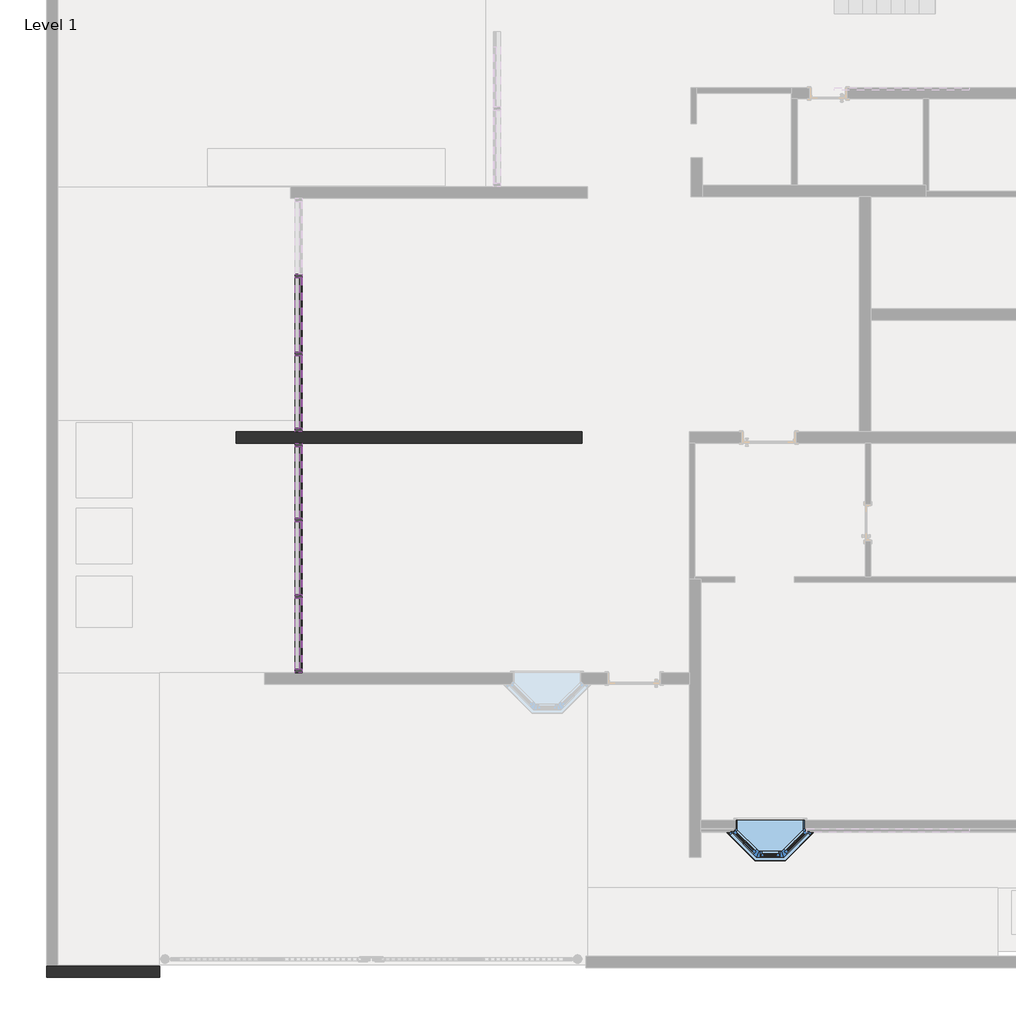
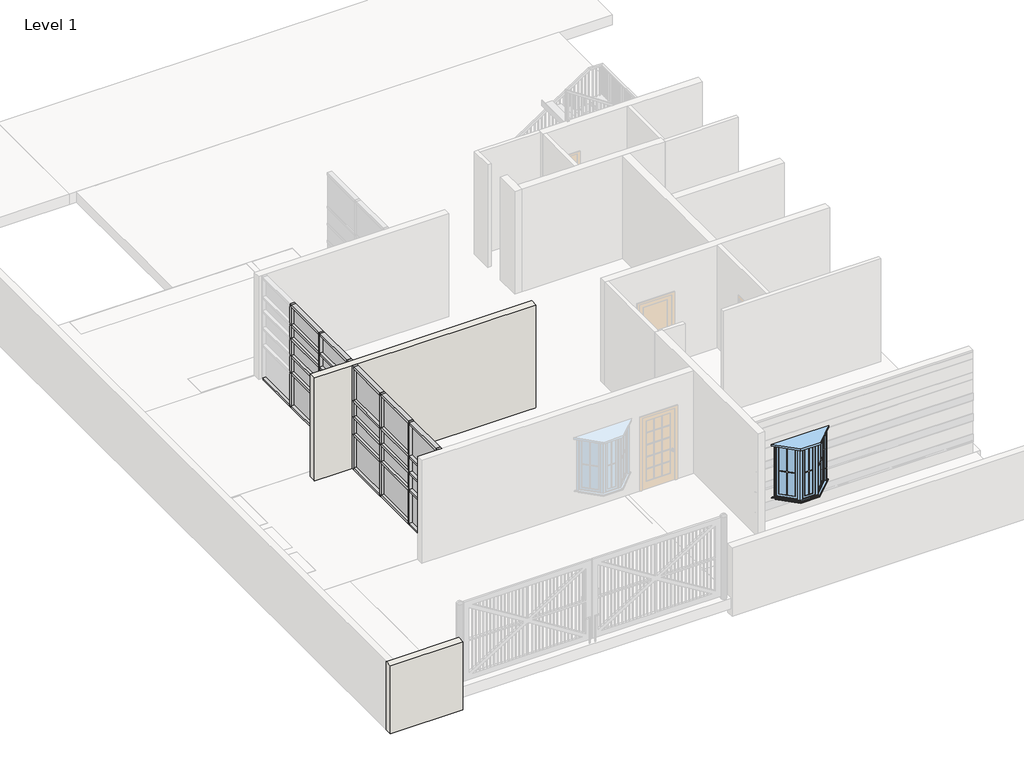
# One storey, part 1 of 5: 59 members, 22 plates, 2 walls, 1 window.
"""IFC4 building model written with IfcOpenShell, lengths in millimetres."""

from ifc_helpers import new_model, si_unit, origin, place, context, project, spatial, faceted_brep, transform, mapped, element, save
from components import member_ace9393b, member_8eff11ef, member_f92b8aa2, member_8e09d03a, member_2b3f0a2a, member_1e564621, member_323df77c, member_86d06fe4, member_556b160f, member_b3098cb3, member_4a65f4ca, member_ce4f90f2, member_13061b82, member_abf390f1, member_37fe5cbd, member_37150780, member_90750a43, member_90c805a2, member_6e77e263, member_47bfaf8a, member_7fd687a9, member_7cfea1b5, system_panel_glazed_a8af599a, system_panel_glazed_c1b4dd64, system_panel_glazed_a0664fa1, system_panel_glazed_cff82037, system_panel_glazed_a94942f9, system_panel_glazed_6f193a35, system_panel_glazed_ac301e25, system_panel_glazed_b1ae2562, system_panel_glazed_b72ced83, system_panel_glazed_3baabbd8, system_panel_glazed_b8338f5c, system_panel_glazed_1cb66d18, system_panel_glazed_2a12a50e, system_panel_glazed_7354da21, system_panel_glazed_2e6a26f2, system_panel_glazed_f09e76d7, window_bay_casement_45_degree_angle_window_4_787d36ed

model = new_model("IFC4")

# Units and contexts
model_context = context("Model", 3, world=origin())
ifc_project = project(units=[si_unit("LENGTHUNIT", "METRE", prefix="MILLI")], contexts=[model_context])

# Site, building, storey
site = spatial("IfcSite", under=ifc_project)
building = spatial("IfcBuilding", under=site)
storey = spatial("IfcBuildingStorey", under=building, Name="Level 1", Elevation=0.0)

# Members
placement = place(None, origin())
member_shape = member_ace9393b(model_context)
element("IfcMember", 1, ObjectType="Rectangular Mullion : 2.5\" x 5\" rectangular", at=placement, inside=storey, context=model_context, shape_type="MappedRepresentation", body=[
    mapped(member_shape, transform((-50759.3380314, -7092.7913973, 3048.0), x_axis=(0.0, 0.0, 1.0), y_axis=(-1.0, 0.0, 0.0), z_axis=(0.0, -1.0, 0.0))),
])
element("IfcMember", 2, ObjectType="Rectangular Mullion : 2.5\" x 5\" rectangular", at=placement, inside=storey, context=model_context, shape_type="MappedRepresentation", body=[
    mapped(member_shape, transform((-50759.3380314, -4381.3413974, 3048.0), x_axis=(0.0, 0.0, 1.0), y_axis=(-1.0, 0.0, 0.0), z_axis=(0.0, -1.0, 0.0))),
])
element("IfcMember", 3, ObjectType="Rectangular Mullion : 2.5\" x 5\" rectangular", at=placement, inside=storey, context=model_context, shape_type="MappedRepresentation", body=[
    mapped(member_shape, transform((-50759.3380314, -3104.9913973, 0.0), x_axis=(0.0, 0.0, -1.0), y_axis=(-1.0, 0.0, 0.0), z_axis=(0.0, 1.0, 0.0))),
])
element("IfcMember", 4, ObjectType="Rectangular Mullion : 2.5\" x 5\" rectangular", at=placement, inside=storey, context=model_context, shape_type="MappedRepresentation", body=[
    mapped(member_shape, transform((-50759.3380314, -5816.4413972, 0.0), x_axis=(0.0, 0.0, -1.0), y_axis=(-1.0, 0.0, 0.0), z_axis=(0.0, 1.0, 0.0))),
])
member_2_shape = member_8eff11ef(model_context)
element("IfcMember", 5, ObjectType="Rectangular Mullion : 2.5\" x 5\" rectangular", at=placement, inside=storey, context=model_context, shape_type="MappedRepresentation", body=[
    mapped(member_2_shape, transform((-50759.3380314, -5752.9413972, 3048.0), x_axis=(0.0, 0.0, 1.0), y_axis=(-1.0, 0.0, 0.0), z_axis=(0.0, -1.0, 0.0))),
])
element("IfcMember", 6, ObjectType="Rectangular Mullion : 2.5\" x 5\" rectangular", at=placement, inside=storey, context=model_context, shape_type="MappedRepresentation", body=[
    mapped(member_2_shape, transform((-50759.3380314, -4444.8413974, 0.0), x_axis=(0.0, 0.0, -1.0), y_axis=(-1.0, 0.0, 0.0), z_axis=(0.0, 1.0, 0.0))),
])
member_3_shape = member_f92b8aa2(model_context)
element("IfcMember", 7, ObjectType="Rectangular Mullion : 2.5\" x 5\" rectangular", at=placement, inside=storey, context=model_context, shape_type="MappedRepresentation", body=[
    mapped(member_3_shape, transform((-50759.3380314, -4413.0913974, 2032.0), x_axis=(0.0, -1.0, 0.0), y_axis=(-1.0, 0.0, 0.0), z_axis=(0.0, 0.0, -1.0))),
])
element("IfcMember", 8, ObjectType="Rectangular Mullion : 2.5\" x 5\" rectangular", at=placement, inside=storey, context=model_context, shape_type="MappedRepresentation", body=[
    mapped(member_3_shape, transform((-50759.3380314, -5784.6913972, 2032.0), x_axis=(0.0, -1.0, 0.0), y_axis=(-1.0, 0.0, 0.0), z_axis=(0.0, 0.0, -1.0))),
])
member_4_shape = member_8e09d03a(model_context)
element("IfcMember", 9, ObjectType="Rectangular Mullion : 2.5\" x 5\" rectangular", at=placement, inside=storey, context=model_context, shape_type="MappedRepresentation", body=[
    mapped(member_4_shape, transform((-50759.3380314, -3041.4913973, 3048.0), x_axis=(0.0, 1.0, 0.0), y_axis=(-1.0, 0.0, 0.0), z_axis=(0.0, 0.0, 1.0))),
])
element("IfcMember", 10, ObjectType="Rectangular Mullion : 2.5\" x 5\" rectangular", at=placement, inside=storey, context=model_context, shape_type="MappedRepresentation", body=[
    mapped(member_4_shape, transform((-50759.3380314, -7156.2913973, 2032.0), x_axis=(0.0, -1.0, 0.0), y_axis=(-1.0, 0.0, 0.0), z_axis=(0.0, 0.0, -1.0))),
])
member_5_shape = member_2b3f0a2a(model_context)
element("IfcMember", 11, ObjectType="Rectangular Mullion : 2.5\" x 5\" rectangular", at=placement, inside=storey, context=model_context, shape_type="MappedRepresentation", body=[
    mapped(member_5_shape, transform((-50759.3380314, -4381.3413974, 2032.0), x_axis=(0.0, 0.0, 1.0), y_axis=(-1.0, 0.0, 0.0), z_axis=(0.0, -1.0, 0.0))),
])
element("IfcMember", 12, ObjectType="Rectangular Mullion : 2.5\" x 5\" rectangular", at=placement, inside=storey, context=model_context, shape_type="MappedRepresentation", body=[
    mapped(member_5_shape, transform((-50759.3380314, -7092.7913973, 2032.0), x_axis=(0.0, 0.0, 1.0), y_axis=(-1.0, 0.0, 0.0), z_axis=(0.0, -1.0, 0.0))),
])
element("IfcMember", 13, ObjectType="Rectangular Mullion : 2.5\" x 5\" rectangular", at=placement, inside=storey, context=model_context, shape_type="MappedRepresentation", body=[
    mapped(member_5_shape, transform((-50759.3380314, -4381.3413974, 1549.4), x_axis=(0.0, 0.0, 1.0), y_axis=(-1.0, 0.0, 0.0), z_axis=(0.0, -1.0, 0.0))),
])
element("IfcMember", 14, ObjectType="Rectangular Mullion : 2.5\" x 5\" rectangular", at=placement, inside=storey, context=model_context, shape_type="MappedRepresentation", body=[
    mapped(member_5_shape, transform((-50759.3380314, -7092.7913973, 1549.4), x_axis=(0.0, 0.0, 1.0), y_axis=(-1.0, 0.0, 0.0), z_axis=(0.0, -1.0, 0.0))),
])
element("IfcMember", 15, ObjectType="Rectangular Mullion : 2.5\" x 5\" rectangular", at=placement, inside=storey, context=model_context, shape_type="MappedRepresentation", body=[
    mapped(member_5_shape, transform((-50759.3380314, -4381.3413974, 1032.9333333), x_axis=(0.0, 0.0, 1.0), y_axis=(-1.0, 0.0, 0.0), z_axis=(0.0, -1.0, 0.0))),
])
element("IfcMember", 16, ObjectType="Rectangular Mullion : 2.5\" x 5\" rectangular", at=placement, inside=storey, context=model_context, shape_type="MappedRepresentation", body=[
    mapped(member_5_shape, transform((-50759.3380314, -7092.7913973, 1032.9333333), x_axis=(0.0, 0.0, 1.0), y_axis=(-1.0, 0.0, 0.0), z_axis=(0.0, -1.0, 0.0))),
])
member_6_shape = member_1e564621(model_context)
element("IfcMember", 17, ObjectType="Rectangular Mullion : 2.5\" x 5\" rectangular", at=placement, inside=storey, context=model_context, shape_type="MappedRepresentation", body=[
    mapped(member_6_shape, transform((-50759.3380314, -5752.9413972, 2032.0), x_axis=(0.0, 0.0, 1.0), y_axis=(-1.0, 0.0, 0.0), z_axis=(0.0, -1.0, 0.0))),
])
element("IfcMember", 18, ObjectType="Rectangular Mullion : 2.5\" x 5\" rectangular", at=placement, inside=storey, context=model_context, shape_type="MappedRepresentation", body=[
    mapped(member_6_shape, transform((-50759.3380314, -5752.9413972, 1549.4), x_axis=(0.0, 0.0, 1.0), y_axis=(-1.0, 0.0, 0.0), z_axis=(0.0, -1.0, 0.0))),
])
element("IfcMember", 19, ObjectType="Rectangular Mullion : 2.5\" x 5\" rectangular", at=placement, inside=storey, context=model_context, shape_type="MappedRepresentation", body=[
    mapped(member_6_shape, transform((-50759.3380314, -5752.9413972, 1032.9333333), x_axis=(0.0, 0.0, 1.0), y_axis=(-1.0, 0.0, 0.0), z_axis=(0.0, -1.0, 0.0))),
])
member_7_shape = member_323df77c(model_context)
element("IfcMember", 20, ObjectType="Rectangular Mullion : 2.5\" x 5\" rectangular", at=placement, inside=storey, context=model_context, shape_type="MappedRepresentation", body=[
    mapped(member_7_shape, transform((-50759.3380314, -4413.0913974, 1549.4), x_axis=(0.0, -1.0, 0.0), y_axis=(-1.0, 0.0, 0.0), z_axis=(0.0, 0.0, -1.0))),
])
element("IfcMember", 21, ObjectType="Rectangular Mullion : 2.5\" x 5\" rectangular", at=placement, inside=storey, context=model_context, shape_type="MappedRepresentation", body=[
    mapped(member_7_shape, transform((-50759.3380314, -5784.6913972, 1549.4), x_axis=(0.0, -1.0, 0.0), y_axis=(-1.0, 0.0, 0.0), z_axis=(0.0, 0.0, -1.0))),
])
member_8_shape = member_86d06fe4(model_context)
element("IfcMember", 22, ObjectType="Rectangular Mullion : 2.5\" x 5\" rectangular", at=placement, inside=storey, context=model_context, shape_type="MappedRepresentation", body=[
    mapped(member_8_shape, transform((-50759.3380314, -3041.4913973, 2032.0), x_axis=(0.0, 1.0, 0.0), y_axis=(-1.0, 0.0, 0.0), z_axis=(0.0, 0.0, 1.0))),
])
element("IfcMember", 23, ObjectType="Rectangular Mullion : 2.5\" x 5\" rectangular", at=placement, inside=storey, context=model_context, shape_type="MappedRepresentation", body=[
    mapped(member_8_shape, transform((-50759.3380314, -7156.2913973, 1549.4), x_axis=(0.0, -1.0, 0.0), y_axis=(-1.0, 0.0, 0.0), z_axis=(0.0, 0.0, -1.0))),
])
member_9_shape = member_556b160f(model_context)
element("IfcMember", 24, ObjectType="Rectangular Mullion : 2.5\" x 5\" rectangular", at=placement, inside=storey, context=model_context, shape_type="MappedRepresentation", body=[
    mapped(member_9_shape, transform((-50759.3380314, -4413.0913974, 0.0), x_axis=(0.0, -1.0, 0.0), y_axis=(-1.0, 0.0, 0.0), z_axis=(0.0, 0.0, -1.0))),
])
element("IfcMember", 25, ObjectType="Rectangular Mullion : 2.5\" x 5\" rectangular", at=placement, inside=storey, context=model_context, shape_type="MappedRepresentation", body=[
    mapped(member_9_shape, transform((-50759.3380314, -5784.6913972, 0.0), x_axis=(0.0, -1.0, 0.0), y_axis=(-1.0, 0.0, 0.0), z_axis=(0.0, 0.0, -1.0))),
])
member_10_shape = member_b3098cb3(model_context)
element("IfcMember", 26, ObjectType="Rectangular Mullion : 2.5\" x 5\" rectangular", at=placement, inside=storey, context=model_context, shape_type="MappedRepresentation", body=[
    mapped(member_10_shape, transform((-50759.3380314, -4413.0913974, 1032.9333333), x_axis=(0.0, -1.0, 0.0), y_axis=(-1.0, 0.0, 0.0), z_axis=(0.0, 0.0, -1.0))),
])
element("IfcMember", 27, ObjectType="Rectangular Mullion : 2.5\" x 5\" rectangular", at=placement, inside=storey, context=model_context, shape_type="MappedRepresentation", body=[
    mapped(member_10_shape, transform((-50759.3380314, -5784.6913972, 1032.9333333), x_axis=(0.0, -1.0, 0.0), y_axis=(-1.0, 0.0, 0.0), z_axis=(0.0, 0.0, -1.0))),
])
member_11_shape = member_4a65f4ca(model_context)
element("IfcMember", 28, ObjectType="Rectangular Mullion : 2.5\" x 5\" rectangular", at=placement, inside=storey, context=model_context, shape_type="MappedRepresentation", body=[
    mapped(member_11_shape, transform((-50759.3380314, -7156.2913973, 0.0), x_axis=(0.0, -1.0, 0.0), y_axis=(-1.0, 0.0, 0.0), z_axis=(0.0, 0.0, -1.0))),
])
member_12_shape = member_ce4f90f2(model_context)
element("IfcMember", 29, ObjectType="Rectangular Mullion : 2.5\" x 5\" rectangular", at=placement, inside=storey, context=model_context, shape_type="MappedRepresentation", body=[
    mapped(member_12_shape, transform((-50759.3380314, -3041.4913973, 1549.4), x_axis=(0.0, 1.0, 0.0), y_axis=(-1.0, 0.0, 0.0), z_axis=(0.0, 0.0, 1.0))),
])
element("IfcMember", 30, ObjectType="Rectangular Mullion : 2.5\" x 5\" rectangular", at=placement, inside=storey, context=model_context, shape_type="MappedRepresentation", body=[
    mapped(member_12_shape, transform((-50759.3380314, -7156.2913973, 1032.9333333), x_axis=(0.0, -1.0, 0.0), y_axis=(-1.0, 0.0, 0.0), z_axis=(0.0, 0.0, -1.0))),
])
element("IfcMember", 31, ObjectType="Rectangular Mullion : 2.5\" x 5\" rectangular", at=placement, inside=storey, context=model_context, shape_type="MappedRepresentation", body=[
    mapped(member_11_shape, transform((-50759.3380314, -3041.4913973, 1032.9333333), x_axis=(0.0, 1.0, 0.0), y_axis=(-1.0, 0.0, 0.0), z_axis=(0.0, 0.0, 1.0))),
])
member_13_shape = member_13061b82(model_context)
element("IfcMember", 32, ObjectType="Rectangular Mullion : 2.5\" x 5\" rectangular", at=placement, inside=storey, context=model_context, shape_type="MappedRepresentation", body=[
    mapped(member_13_shape, transform((-50759.3380314, -1473.0413972, 3048.0), x_axis=(0.0, 0.0, 1.0), y_axis=(1.0, 0.0, 0.0), z_axis=(0.0, 1.0, 0.0))),
])
element("IfcMember", 33, ObjectType="Rectangular Mullion : 2.5\" x 5\" rectangular", at=placement, inside=storey, context=model_context, shape_type="MappedRepresentation", body=[
    mapped(member_13_shape, transform((-50759.3380314, -2774.7913973, 0.0), x_axis=(0.0, 0.0, -1.0), y_axis=(1.0, 0.0, 0.0), z_axis=(0.0, -1.0, 0.0))),
])
element("IfcMember", 34, ObjectType="Rectangular Mullion : 2.5\" x 5\" rectangular", at=placement, inside=storey, context=model_context, shape_type="MappedRepresentation", body=[
    mapped(member_13_shape, transform((-50759.3380314, -12.5413974, 0.0), x_axis=(0.0, 0.0, -1.0), y_axis=(1.0, 0.0, 0.0), z_axis=(0.0, -1.0, 0.0))),
])
member_14_shape = member_abf390f1(model_context)
element("IfcMember", 35, ObjectType="Rectangular Mullion : 2.5\" x 5\" rectangular", at=placement, inside=storey, context=model_context, shape_type="MappedRepresentation", body=[
    mapped(member_14_shape, transform((-50759.3380314, -76.0413974, 3048.0), x_axis=(0.0, 0.0, 1.0), y_axis=(1.0, 0.0, 0.0), z_axis=(0.0, 1.0, 0.0))),
])
element("IfcMember", 36, ObjectType="Rectangular Mullion : 2.5\" x 5\" rectangular", at=placement, inside=storey, context=model_context, shape_type="MappedRepresentation", body=[
    mapped(member_14_shape, transform((-50759.3380314, -1409.5413972, 0.0), x_axis=(0.0, 0.0, -1.0), y_axis=(1.0, 0.0, 0.0), z_axis=(0.0, -1.0, 0.0))),
])
element("IfcMember", 37, ObjectType="Rectangular Mullion : 2.5\" x 5\" rectangular", at=placement, inside=storey, context=model_context, shape_type="MappedRepresentation", body=[
    mapped(member_3_shape, transform((-50759.3380314, -1441.2913972, 0.0), x_axis=(0.0, 1.0, 0.0), y_axis=(1.0, 0.0, 0.0), z_axis=(0.0, 0.0, -1.0))),
])
element("IfcMember", 38, ObjectType="Rectangular Mullion : 2.5\" x 5\" rectangular", at=placement, inside=storey, context=model_context, shape_type="MappedRepresentation", body=[
    mapped(member_3_shape, transform((-50759.3380314, -44.2913974, 0.0), x_axis=(0.0, 1.0, 0.0), y_axis=(1.0, 0.0, 0.0), z_axis=(0.0, 0.0, -1.0))),
])
member_15_shape = member_37fe5cbd(model_context)
element("IfcMember", 39, ObjectType="Rectangular Mullion : 2.5\" x 5\" rectangular", at=placement, inside=storey, context=model_context, shape_type="MappedRepresentation", body=[
    mapped(member_15_shape, transform((-50759.3380314, -1473.0413972, 1016.0), x_axis=(0.0, 0.0, 1.0), y_axis=(1.0, 0.0, 0.0), z_axis=(0.0, 1.0, 0.0))),
])
element("IfcMember", 40, ObjectType="Rectangular Mullion : 2.5\" x 5\" rectangular", at=placement, inside=storey, context=model_context, shape_type="MappedRepresentation", body=[
    mapped(member_15_shape, transform((-50759.3380314, -1473.0413972, 2032.0), x_axis=(0.0, 0.0, 1.0), y_axis=(1.0, 0.0, 0.0), z_axis=(0.0, 1.0, 0.0))),
])
element("IfcMember", 41, ObjectType="Rectangular Mullion : 2.5\" x 5\" rectangular", at=placement, inside=storey, context=model_context, shape_type="MappedRepresentation", body=[
    mapped(member_15_shape, transform((-50759.3380314, -1473.0413972, 1524.0), x_axis=(0.0, 0.0, 1.0), y_axis=(1.0, 0.0, 0.0), z_axis=(0.0, 1.0, 0.0))),
])
element("IfcMember", 42, ObjectType="Rectangular Mullion : 2.5\" x 5\" rectangular", at=placement, inside=storey, context=model_context, shape_type="MappedRepresentation", body=[
    mapped(member_15_shape, transform((-50759.3380314, -1473.0413972, 2438.4), x_axis=(0.0, 0.0, 1.0), y_axis=(1.0, 0.0, 0.0), z_axis=(0.0, 1.0, 0.0))),
])
member_16_shape = member_37150780(model_context)
element("IfcMember", 43, ObjectType="Rectangular Mullion : 2.5\" x 5\" rectangular", at=placement, inside=storey, context=model_context, shape_type="MappedRepresentation", body=[
    mapped(member_16_shape, transform((-50759.3380314, -76.0413974, 1016.0), x_axis=(0.0, 0.0, 1.0), y_axis=(1.0, 0.0, 0.0), z_axis=(0.0, 1.0, 0.0))),
])
element("IfcMember", 44, ObjectType="Rectangular Mullion : 2.5\" x 5\" rectangular", at=placement, inside=storey, context=model_context, shape_type="MappedRepresentation", body=[
    mapped(member_16_shape, transform((-50759.3380314, -76.0413974, 2032.0), x_axis=(0.0, 0.0, 1.0), y_axis=(1.0, 0.0, 0.0), z_axis=(0.0, 1.0, 0.0))),
])
element("IfcMember", 45, ObjectType="Rectangular Mullion : 2.5\" x 5\" rectangular", at=placement, inside=storey, context=model_context, shape_type="MappedRepresentation", body=[
    mapped(member_16_shape, transform((-50759.3380314, -76.0413974, 1524.0), x_axis=(0.0, 0.0, 1.0), y_axis=(1.0, 0.0, 0.0), z_axis=(0.0, 1.0, 0.0))),
])
element("IfcMember", 46, ObjectType="Rectangular Mullion : 2.5\" x 5\" rectangular", at=placement, inside=storey, context=model_context, shape_type="MappedRepresentation", body=[
    mapped(member_16_shape, transform((-50759.3380314, -76.0413974, 2438.4), x_axis=(0.0, 0.0, 1.0), y_axis=(1.0, 0.0, 0.0), z_axis=(0.0, 1.0, 0.0))),
])
member_17_shape = member_90750a43(model_context)
element("IfcMember", 47, ObjectType="Rectangular Mullion : 2.5\" x 5\" rectangular", at=placement, inside=storey, context=model_context, shape_type="MappedRepresentation", body=[
    mapped(member_17_shape, transform((-50759.3380314, -1441.2913972, 1016.0), x_axis=(0.0, 1.0, 0.0), y_axis=(1.0, 0.0, 0.0), z_axis=(0.0, 0.0, -1.0))),
])
element("IfcMember", 48, ObjectType="Rectangular Mullion : 2.5\" x 5\" rectangular", at=placement, inside=storey, context=model_context, shape_type="MappedRepresentation", body=[
    mapped(member_17_shape, transform((-50759.3380314, -44.2913974, 1016.0), x_axis=(0.0, 1.0, 0.0), y_axis=(1.0, 0.0, 0.0), z_axis=(0.0, 0.0, -1.0))),
])
element("IfcMember", 49, ObjectType="Rectangular Mullion : 2.5\" x 5\" rectangular", at=placement, inside=storey, context=model_context, shape_type="MappedRepresentation", body=[
    mapped(member_17_shape, transform((-50759.3380314, -1441.2913972, 1524.0), x_axis=(0.0, 1.0, 0.0), y_axis=(1.0, 0.0, 0.0), z_axis=(0.0, 0.0, -1.0))),
])
element("IfcMember", 50, ObjectType="Rectangular Mullion : 2.5\" x 5\" rectangular", at=placement, inside=storey, context=model_context, shape_type="MappedRepresentation", body=[
    mapped(member_17_shape, transform((-50759.3380314, -44.2913974, 1524.0), x_axis=(0.0, 1.0, 0.0), y_axis=(1.0, 0.0, 0.0), z_axis=(0.0, 0.0, -1.0))),
])
member_18_shape = member_90c805a2(model_context)
element("IfcMember", 51, ObjectType="Rectangular Mullion : 2.5\" x 5\" rectangular", at=placement, inside=storey, context=model_context, shape_type="MappedRepresentation", body=[
    mapped(member_18_shape, transform((-50759.3380314, -1441.2913972, 2032.0), x_axis=(0.0, 1.0, 0.0), y_axis=(1.0, 0.0, 0.0), z_axis=(0.0, 0.0, -1.0))),
])
element("IfcMember", 52, ObjectType="Rectangular Mullion : 2.5\" x 5\" rectangular", at=placement, inside=storey, context=model_context, shape_type="MappedRepresentation", body=[
    mapped(member_18_shape, transform((-50759.3380314, -44.2913974, 2032.0), x_axis=(0.0, 1.0, 0.0), y_axis=(1.0, 0.0, 0.0), z_axis=(0.0, 0.0, -1.0))),
])
member_19_shape = member_6e77e263(model_context)
element("IfcMember", 53, ObjectType="Rectangular Mullion : 2.5\" x 5\" rectangular", at=placement, inside=storey, context=model_context, shape_type="MappedRepresentation", body=[
    mapped(member_19_shape, transform((-50759.3380314, -1441.2913972, 2438.4), x_axis=(0.0, 1.0, 0.0), y_axis=(1.0, 0.0, 0.0), z_axis=(0.0, 0.0, -1.0))),
])
element("IfcMember", 54, ObjectType="Rectangular Mullion : 2.5\" x 5\" rectangular", at=placement, inside=storey, context=model_context, shape_type="MappedRepresentation", body=[
    mapped(member_19_shape, transform((-50759.3380314, -44.2913974, 2438.4), x_axis=(0.0, 1.0, 0.0), y_axis=(1.0, 0.0, 0.0), z_axis=(0.0, 0.0, -1.0))),
])
member_20_shape = member_47bfaf8a(model_context)
element("IfcMember", 55, ObjectType="Rectangular Mullion : 2.5\" x 5\" rectangular", at=placement, inside=storey, context=model_context, shape_type="MappedRepresentation", body=[
    mapped(member_20_shape, transform((-50759.3380314, -2838.2913973, 3048.0), x_axis=(0.0, -1.0, 0.0), y_axis=(1.0, 0.0, 0.0), z_axis=(0.0, 0.0, 1.0))),
])
element("IfcMember", 56, ObjectType="Rectangular Mullion : 2.5\" x 5\" rectangular", at=placement, inside=storey, context=model_context, shape_type="MappedRepresentation", body=[
    mapped(member_4_shape, transform((-50759.3380314, -2838.2913973, 1016.0), x_axis=(0.0, -1.0, 0.0), y_axis=(1.0, 0.0, 0.0), z_axis=(0.0, 0.0, 1.0))),
])
member_21_shape = member_7fd687a9(model_context)
element("IfcMember", 57, ObjectType="Rectangular Mullion : 2.5\" x 5\" rectangular", at=placement, inside=storey, context=model_context, shape_type="MappedRepresentation", body=[
    mapped(member_21_shape, transform((-50759.3380314, -2838.2913973, 2032.0), x_axis=(0.0, -1.0, 0.0), y_axis=(1.0, 0.0, 0.0), z_axis=(0.0, 0.0, 1.0))),
])
element("IfcMember", 58, ObjectType="Rectangular Mullion : 2.5\" x 5\" rectangular", at=placement, inside=storey, context=model_context, shape_type="MappedRepresentation", body=[
    mapped(member_21_shape, transform((-50759.3380314, -2838.2913973, 1524.0), x_axis=(0.0, -1.0, 0.0), y_axis=(1.0, 0.0, 0.0), z_axis=(0.0, 0.0, 1.0))),
])
member_22_shape = member_7cfea1b5(model_context)
element("IfcMember", 59, ObjectType="Rectangular Mullion : 2.5\" x 5\" rectangular", at=placement, inside=storey, context=model_context, shape_type="MappedRepresentation", body=[
    mapped(member_22_shape, transform((-50759.3380314, -2838.2913973, 2438.4), x_axis=(0.0, -1.0, 0.0), y_axis=(1.0, 0.0, 0.0), z_axis=(0.0, 0.0, 1.0))),
])

# Plates
system_panel_glazed_shape = system_panel_glazed_a8af599a(model_context)
element("IfcPlate", 60, ObjectType="System Panel : Glazed", at=placement, inside=storey, context=model_context, shape_type="MappedRepresentation", body=[
    mapped(system_panel_glazed_shape, transform((-50759.3380314, -3743.1663973, 2063.75), x_axis=(0.0, -1.0, 0.0), y_axis=(1.0, 0.0, 0.0), z_axis=(0.0, 0.0, 1.0))),
])
element("IfcPlate", 61, ObjectType="System Panel : Glazed", at=placement, inside=storey, context=model_context, shape_type="MappedRepresentation", body=[
    mapped(system_panel_glazed_shape, transform((-50759.3380314, -6454.6163972, 2063.75), x_axis=(0.0, -1.0, 0.0), y_axis=(1.0, 0.0, 0.0), z_axis=(0.0, 0.0, 1.0))),
])
system_panel_glazed_2_shape = system_panel_glazed_c1b4dd64(model_context)
element("IfcPlate", 62, ObjectType="System Panel : Glazed", at=placement, inside=storey, context=model_context, shape_type="MappedRepresentation", body=[
    mapped(system_panel_glazed_2_shape, transform((-50759.3380314, -5098.8913973, 2063.75), x_axis=(0.0, -1.0, 0.0), y_axis=(1.0, 0.0, 0.0), z_axis=(0.0, 0.0, 1.0))),
])
system_panel_glazed_3_shape = system_panel_glazed_a0664fa1(model_context)
element("IfcPlate", 63, ObjectType="System Panel : Glazed", at=placement, inside=storey, context=model_context, shape_type="MappedRepresentation", body=[
    mapped(system_panel_glazed_3_shape, transform((-50759.3380314, -3743.1663973, 1581.15), x_axis=(0.0, -1.0, 0.0), y_axis=(1.0, 0.0, 0.0), z_axis=(0.0, 0.0, 1.0))),
])
element("IfcPlate", 64, ObjectType="System Panel : Glazed", at=placement, inside=storey, context=model_context, shape_type="MappedRepresentation", body=[
    mapped(system_panel_glazed_3_shape, transform((-50759.3380314, -6454.6163972, 1581.15), x_axis=(0.0, -1.0, 0.0), y_axis=(1.0, 0.0, 0.0), z_axis=(0.0, 0.0, 1.0))),
])
system_panel_glazed_4_shape = system_panel_glazed_cff82037(model_context)
element("IfcPlate", 65, ObjectType="System Panel : Glazed", at=placement, inside=storey, context=model_context, shape_type="MappedRepresentation", body=[
    mapped(system_panel_glazed_4_shape, transform((-50759.3380314, -5098.8913973, 1581.15), x_axis=(0.0, -1.0, 0.0), y_axis=(1.0, 0.0, 0.0), z_axis=(0.0, 0.0, 1.0))),
])
system_panel_glazed_5_shape = system_panel_glazed_a94942f9(model_context)
element("IfcPlate", 66, ObjectType="System Panel : Glazed", at=placement, inside=storey, context=model_context, shape_type="MappedRepresentation", body=[
    mapped(system_panel_glazed_5_shape, transform((-50759.3380314, -3743.1663973, 63.5), x_axis=(0.0, -1.0, 0.0), y_axis=(1.0, 0.0, 0.0), z_axis=(0.0, 0.0, 1.0))),
])
element("IfcPlate", 67, ObjectType="System Panel : Glazed", at=placement, inside=storey, context=model_context, shape_type="MappedRepresentation", body=[
    mapped(system_panel_glazed_5_shape, transform((-50759.3380314, -6454.6163972, 63.5), x_axis=(0.0, -1.0, 0.0), y_axis=(1.0, 0.0, 0.0), z_axis=(0.0, 0.0, 1.0))),
])
system_panel_glazed_6_shape = system_panel_glazed_6f193a35(model_context)
element("IfcPlate", 68, ObjectType="System Panel : Glazed", at=placement, inside=storey, context=model_context, shape_type="MappedRepresentation", body=[
    mapped(system_panel_glazed_6_shape, transform((-50759.3380314, -5098.8913973, 63.5), x_axis=(0.0, -1.0, 0.0), y_axis=(1.0, 0.0, 0.0), z_axis=(0.0, 0.0, 1.0))),
])
system_panel_glazed_7_shape = system_panel_glazed_ac301e25(model_context)
element("IfcPlate", 69, ObjectType="System Panel : Glazed", at=placement, inside=storey, context=model_context, shape_type="MappedRepresentation", body=[
    mapped(system_panel_glazed_7_shape, transform((-50759.3380314, -3743.1663973, 1064.6833333), x_axis=(0.0, -1.0, 0.0), y_axis=(1.0, 0.0, 0.0), z_axis=(0.0, 0.0, 1.0))),
])
element("IfcPlate", 70, ObjectType="System Panel : Glazed", at=placement, inside=storey, context=model_context, shape_type="MappedRepresentation", body=[
    mapped(system_panel_glazed_7_shape, transform((-50759.3380314, -6454.6163972, 1064.6833333), x_axis=(0.0, -1.0, 0.0), y_axis=(1.0, 0.0, 0.0), z_axis=(0.0, 0.0, 1.0))),
])
system_panel_glazed_8_shape = system_panel_glazed_b1ae2562(model_context)
element("IfcPlate", 71, ObjectType="System Panel : Glazed", at=placement, inside=storey, context=model_context, shape_type="MappedRepresentation", body=[
    mapped(system_panel_glazed_8_shape, transform((-50759.3380314, -5098.8913973, 1064.6833333), x_axis=(0.0, -1.0, 0.0), y_axis=(1.0, 0.0, 0.0), z_axis=(0.0, 0.0, 1.0))),
])
system_panel_glazed_9_shape = system_panel_glazed_b72ced83(model_context)
element("IfcPlate", 72, ObjectType="System Panel : Glazed", at=placement, inside=storey, context=model_context, shape_type="MappedRepresentation", body=[
    mapped(system_panel_glazed_9_shape, transform((-50759.3380314, -2123.9163972, 63.5), x_axis=(0.0, 1.0, 0.0), y_axis=(-1.0, 0.0, 0.0), z_axis=(0.0, 0.0, 1.0))),
])
system_panel_glazed_10_shape = system_panel_glazed_3baabbd8(model_context)
element("IfcPlate", 73, ObjectType="System Panel : Glazed", at=placement, inside=storey, context=model_context, shape_type="MappedRepresentation", body=[
    mapped(system_panel_glazed_10_shape, transform((-50759.3380314, -742.7913973, 63.5), x_axis=(0.0, 1.0, 0.0), y_axis=(-1.0, 0.0, 0.0), z_axis=(0.0, 0.0, 1.0))),
])
system_panel_glazed_11_shape = system_panel_glazed_b8338f5c(model_context)
element("IfcPlate", 74, ObjectType="System Panel : Glazed", at=placement, inside=storey, context=model_context, shape_type="MappedRepresentation", body=[
    mapped(system_panel_glazed_11_shape, transform((-50759.3380314, -2123.9163972, 1047.75), x_axis=(0.0, 1.0, 0.0), y_axis=(-1.0, 0.0, 0.0), z_axis=(0.0, 0.0, 1.0))),
])
element("IfcPlate", 75, ObjectType="System Panel : Glazed", at=placement, inside=storey, context=model_context, shape_type="MappedRepresentation", body=[
    mapped(system_panel_glazed_11_shape, transform((-50759.3380314, -2123.9163972, 1555.75), x_axis=(0.0, 1.0, 0.0), y_axis=(-1.0, 0.0, 0.0), z_axis=(0.0, 0.0, 1.0))),
])
system_panel_glazed_12_shape = system_panel_glazed_1cb66d18(model_context)
element("IfcPlate", 76, ObjectType="System Panel : Glazed", at=placement, inside=storey, context=model_context, shape_type="MappedRepresentation", body=[
    mapped(system_panel_glazed_12_shape, transform((-50759.3380314, -742.7913973, 1047.75), x_axis=(0.0, 1.0, 0.0), y_axis=(-1.0, 0.0, 0.0), z_axis=(0.0, 0.0, 1.0))),
])
element("IfcPlate", 77, ObjectType="System Panel : Glazed", at=placement, inside=storey, context=model_context, shape_type="MappedRepresentation", body=[
    mapped(system_panel_glazed_12_shape, transform((-50759.3380314, -742.7913973, 1555.75), x_axis=(0.0, 1.0, 0.0), y_axis=(-1.0, 0.0, 0.0), z_axis=(0.0, 0.0, 1.0))),
])
system_panel_glazed_13_shape = system_panel_glazed_2a12a50e(model_context)
element("IfcPlate", 78, ObjectType="System Panel : Glazed", at=placement, inside=storey, context=model_context, shape_type="MappedRepresentation", body=[
    mapped(system_panel_glazed_13_shape, transform((-50759.3380314, -2123.9163972, 2063.75), x_axis=(0.0, 1.0, 0.0), y_axis=(-1.0, 0.0, 0.0), z_axis=(0.0, 0.0, 1.0))),
])
system_panel_glazed_14_shape = system_panel_glazed_7354da21(model_context)
element("IfcPlate", 79, ObjectType="System Panel : Glazed", at=placement, inside=storey, context=model_context, shape_type="MappedRepresentation", body=[
    mapped(system_panel_glazed_14_shape, transform((-50759.3380314, -742.7913973, 2063.75), x_axis=(0.0, 1.0, 0.0), y_axis=(-1.0, 0.0, 0.0), z_axis=(0.0, 0.0, 1.0))),
])
system_panel_glazed_15_shape = system_panel_glazed_2e6a26f2(model_context)
element("IfcPlate", 80, ObjectType="System Panel : Glazed", at=placement, inside=storey, context=model_context, shape_type="MappedRepresentation", body=[
    mapped(system_panel_glazed_15_shape, transform((-50759.3380314, -2123.9163972, 2470.15), x_axis=(0.0, 1.0, 0.0), y_axis=(-1.0, 0.0, 0.0), z_axis=(0.0, 0.0, 1.0))),
])
system_panel_glazed_16_shape = system_panel_glazed_f09e76d7(model_context)
element("IfcPlate", 81, ObjectType="System Panel : Glazed", at=placement, inside=storey, context=model_context, shape_type="MappedRepresentation", body=[
    mapped(system_panel_glazed_16_shape, transform((-50759.3380314, -742.7913973, 2470.15), x_axis=(0.0, 1.0, 0.0), y_axis=(-1.0, 0.0, 0.0), z_axis=(0.0, 0.0, 1.0))),
])

# Walls
element("IfcWall", 82, ObjectType="OUTER WALL 8\"", at=placement, inside=storey, context=model_context, shape_type="Brep", body=[
    faceted_brep([(-45679.3380314, -2838.2913973, 0.0), (-50556.1380314, -2838.2913973, 0.0), (-50759.3380314, -2838.2913973, 0.0), (-51880.9582963, -2838.2913973, 0.0), (-51880.9582963, -2838.2913973, 3048.0), (-50759.3380314, -2838.2913973, 3048.0), (-50556.1380314, -2838.2913973, 3048.0), (-45679.3380314, -2838.2913973, 3048.0), (-45679.3380314, -3041.4913973, 0.0), (-45679.3380314, -3041.4913973, 3048.0), (-50556.1380314, -3041.4913973, 3048.0), (-50759.3380314, -3041.4913973, 3048.0), (-51880.9582963, -3041.4913973, 3048.0), (-51880.9582963, -3041.4913973, 0.0), (-50759.3380314, -3041.4913973, 0.0), (-50556.1380314, -3041.4913973, 0.0)], [[[0, 1, 2, 3, 4, 5, 6, 7]], [[8, 9, 10, 11, 12, 13, 14, 15]], [[3, 2, 1, 0, 8, 15, 14, 13]], [[4, 3, 13, 12]], [[7, 6, 5, 4, 12, 11, 10, 9]], [[0, 7, 9, 8]]]),
])
element("IfcWall", 83, ObjectType="OUTER WALL 8\"", at=placement, inside=storey, context=model_context, shape_type="Brep", body=[
    faceted_brep([(-53248.5380314, -12412.3889249, -499.9883677), (-55279.4412112, -12412.3889249, -499.9883677), (-55279.4412112, -12412.3889249, 1524.0), (-55076.2412112, -12412.3889249, 1524.0), (-53248.5380314, -12412.3889249, 1524.0), (-53248.5380314, -12615.5889249, -499.9883677), (-53248.5380314, -12615.5889249, 1524.0), (-55279.4412112, -12615.5889249, 1524.0), (-55279.4412112, -12615.5889249, -499.9883677)], [[[0, 1, 2, 3, 4]], [[5, 6, 7, 8]], [[1, 0, 5, 8]], [[4, 3, 2, 7, 6]], [[0, 4, 6, 5]], [[2, 1, 8, 7]]]),
])

# Window
window_bay_casement_45_degree_angle_window_4_shape = window_bay_casement_45_degree_angle_window_4_787d36ed(model_context)
element("IfcWindow", 84, ObjectType="Window-Bay-Casement-45_Degree_Angle : WINDOW 4'", at=placement, inside=storey, context=model_context, shape_type="MappedRepresentation", body=[
    mapped(window_bay_casement_45_degree_angle_window_4_shape, transform((-42301.1380314, -9899.4913973, 0.0), x_axis=(-1.0, 0.0, 0.0), y_axis=(0.0, -1.0, 0.0), z_axis=(0.0, 0.0, 1.0))),
])

save(model, "model.ifc")

# Revit data of these elements
# Type "Rectangular Mullion : 2.5\" x 5\" rectangular"
#   built-in parameter 1007304 = 0.416667 (stored number, unit not read)
#   built-in parameter 1007301 = 0.104167 (stored number, unit not read)
#   built-in parameter 1007300 = 0.104167 (stored number, unit not read)
# Type "System Panel : Glazed"
#   Construction Type Id = "GSP4R"
#   Analytic Construction = "1/8 in Pilkington single glazing"
#   Visual Light Transmittance = 0.9
#   Solar Heat Gain Coefficient = 0.86
#   Heat Transfer Coefficient (U) = 1.18115 BTU/(h·ft²·°F)
#   Define Thermal Properties by = 1
# Type "OUTER WALL 8\""
#   Assembly Code = "B2010"
#   Layers, outside or top first: 0' - 8" "BEIGE COLOUR" (function 1)
# Type "Window-Bay-Casement-45_Degree_Angle : WINDOW 4'"
#   Type Mark = "19"
#   Fire Rating = "0.5h"
#   Assembly Code = "B2020100"
#   Analytic Construction = "Double glazing - domestic"
#   Width of Middle Sash = 1' - 2.38909"
#   Width = 4' - 0"
#   Visual Light Transmittance = 0.81
#   Thermal Resistance (R) = 1.8146 (h·ft²·°F)/BTU
#   Solar Heat Gain Coefficient = 0.76
#   Rough Width = 4' - 0 1/2"
#   Rough Height = 5' - 0 1/2"
#   Length 4 = 0' - 1.13909"
#   Length 3 = 0' - 0.51777"
#   Length 2 = 1' - 7.42462"
#   Length 1 = 1' - 2.80546"
#   Wall Thickness [instance default] = 0' - 6"
#   Trim Width = 4' - 5.03553"
#   Trim Height = 5' - 0"
#   Height 1 = 5' - 2"
#   Height = 5' - 0"
#   Heat Transfer Coefficient (U) = 0.5511 BTU/(h·ft²·°F)
#   Depth = 1' - 6"
#   Default Sill Height = 2' - 0"
#   Angle 1 = 22.50°
#   Angle = 45.00°
#   Center Muntin Visibility = yes
#   Side Muntin Visibility = yes
#   Interior Trim Visibility [instance default] = yes
#   Exterior Trim Visibility [instance default] = yes
#   Center Muntin Pattern = Muntin Pattern_2x2 : Muntin Pattern_2x2
#   Side Muntin Pattern = Muntin Pattern_2x2 : Muntin Pattern_2x2
#   Interior Trim Material = Wood - Stained
#   Exterior Trim Material = Clad - White
#   Exterior Trim = element 406231
#   Interior Trim = Trim-Window-Interior-Flat : Picture Frame
#   Interior Frame Material = Wood - Stained
#   Glass Panel Material = Glass
#   Exterior Frame Material = Clad - White
#   Wall Closure = (empty or 0)
# Elements 1, 2, 3, 4, 5, 6, 7, 8, 9, 10, 11, 12, 13, 14, 15, 16, 17, 18, 19, 20, 21, 22, 23, 24, 25, 26, 27, 28, 29, 30, 31, 32, 33, 34, 35, 36, 37, 38, 39, 40, 41, 42, 43, 44, 45, 46, 47, 48, 49, 50, 51, 52, 53, 54, 55, 56, 57, 58, 59 (IfcMember, "Rectangular Mullion : 2.5\" x 5\" rectangular")
#   Phase Created = New Construction
#   Materials on its faces: "Aluminum"
# Elements 60, 61, 62, 63, 64, 65, 66, 67, 68, 69, 70, 71, 72, 73, 74, 75, 76, 77, 78, 79, 80, 81 (IfcPlate, "System Panel : Glazed")
#   Phase Created = New Construction
#   Materials on its faces: "glass panel 223"
# Element 82 (IfcWall, "OUTER WALL 8\"")
#   Top Offset = 0' - 0"
#   Base Offset = 0' - 0"
#   wall height = 10' - 0"
#   Phase Created = New Construction
#   Base Constraint = Level 1
#   Top Constraint = Level 2
#   Materials on its faces: "BEIGE COLOUR"
# Element 83 (IfcWall, "OUTER WALL 8\"")
#   built-in parameter 1001111 = -1' - 7.68458"
#   Top Offset = 0' - 0"
#   Base Offset = -1' - 7.68458"
#   Unconnected Height = 6' - 7.68458"
#   wall height = 6' - 7.68458"
#   Phase Created = New Construction
#   Base Constraint = Level 1
#   Materials on its faces: "BEIGE COLOUR"
# Element 84 (IfcWindow, "Window-Bay-Casement-45_Degree_Angle : WINDOW 4'")
#   Mark = "3"
#   Interior Trim Visibility = yes
#   Exterior Trim Visibility = yes
#   Phase Created = New Construction
#   Materials on its faces: "Wood - Stained", "Clad - White", "Glass"
# Materials
#   "BEIGE COLOUR": class "Generic", colour RGB 120 120 120, transparency 0, Cost = 0
#   "Wood - Stained": class "Wood", colour RGB 224 178 126, transparency 0, Cost = 0
#   "Clad - White": class "Wood", colour RGB 242 242 238, transparency 0, Cost = 0
#   "Glass": class "Glass", colour RGB 0 128 192, transparency 0.75, Description = "Soda Lime Glass", Cost = 0
#   "Aluminum": class "Metal", colour RGB 247 247 247, transparency 0, Description = "Aluminum 6061", Cost = 0
#   "glass panel 223": class "Generic", colour RGB 120 120 120, transparency 0, Cost = 0
# Room at (-38973.738, -1834.991) mm, phase "New Construction", upper level "Level 1", upper offset 10' - 0", lower offset 0' - 0"
#   Number = "1"
#   Name = "Room"
# Room at (-38973.738, 374.809) mm, phase "New Construction", upper level "Level 1", upper offset 10' - 0", lower offset 0' - 0"
#   Number = "2"
#   Name = "Room"
# Room at (-38427.638, 2330.609) mm, phase "New Construction", upper level "Level 1", upper offset 10' - 0", lower offset 0' - 0"
#   Number = "3"
#   Name = "Room"
# Room at (-40688.238, 2356.009) mm, phase "New Construction", upper level "Level 1", upper offset 10' - 0", lower offset 0' - 0"
#   Number = "4"
#   Name = "Room"
# Room at (-38008.538, 4553.109) mm, phase "New Construction", upper level "Level 1", upper offset 10' - 0", lower offset 0' - 0"
#   Number = "5"
#   Name = "Room"
# Room at (-38948.338, -4209.891) mm, phase "New Construction", upper level "Level 1", upper offset 10' - 0", lower offset 0' - 0"
#   Number = "6"
#   Name = "Room"
# Room at (-40523.138, -6419.691) mm, phase "New Construction", upper level "Level 1", upper offset 10' - 0", lower offset 0' - 0"
#   Number = "7"
#   Name = "Room"
# Room at (-38440.338, 6762.909) mm, phase "New Construction", upper level "Level 1", upper offset 10' - 0", lower offset 0' - 0"
#   Number = "8"
#   Name = "Room"
# Room at (-44053.738, 1543.209) mm, phase "New Construction", upper level "Level 1", upper offset 10' - 0", lower offset 0' - 0"
#   Number = "9"
#   Name = "Room"
